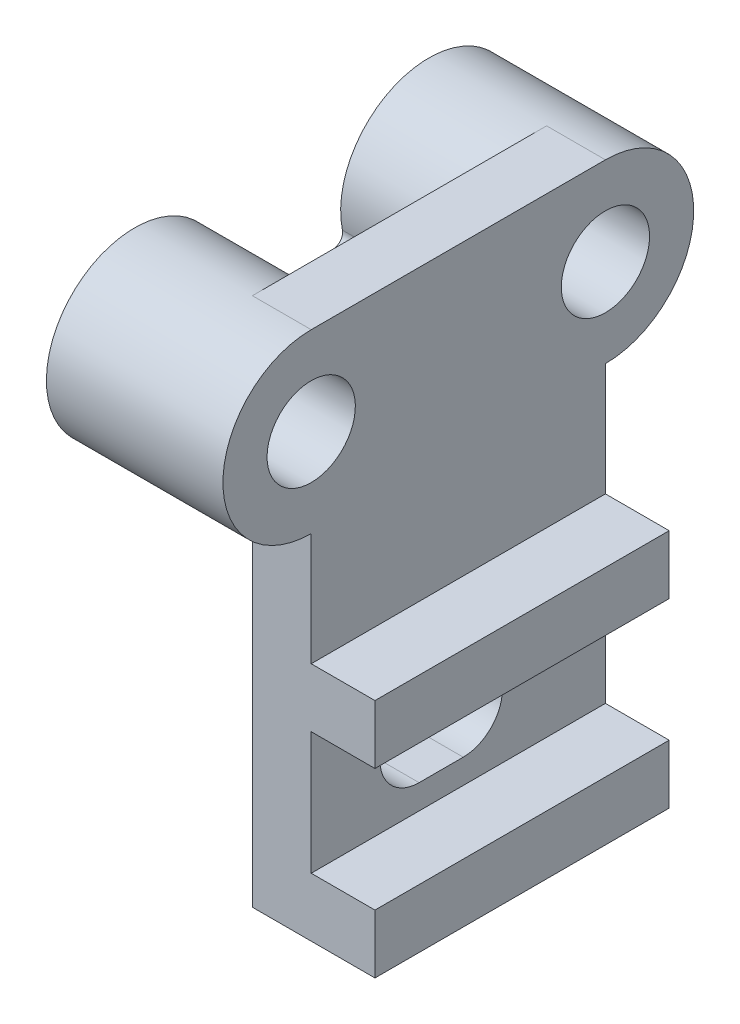
ISO-10303-21;
HEADER;
FILE_DESCRIPTION(('STEP AP214'),'2;1');
FILE_NAME('part.step','',(''),(''),'','','');
FILE_SCHEMA(('AUTOMOTIVE_DESIGN { 1 0 10303 214 1 1 1 1 }'));
ENDSEC;
DATA;
#1=APPLICATION_CONTEXT('core data for automotive mechanical design processes');
#2=APPLICATION_PROTOCOL_DEFINITION('international standard','automotive_design',2000,#1);
#3=PRODUCT_CONTEXT('',#1,'mechanical');
#4=PRODUCT('Part','Part','',(#3));
#5=PRODUCT_RELATED_PRODUCT_CATEGORY('part','',(#4));
#6=PRODUCT_DEFINITION_FORMATION('','',#4);
#7=PRODUCT_DEFINITION_CONTEXT('part definition',#1,'design');
#8=PRODUCT_DEFINITION('design','',#6,#7);
#9=PRODUCT_DEFINITION_SHAPE('','',#8);
#10=(LENGTH_UNIT() NAMED_UNIT(*) SI_UNIT(.MILLI.,.METRE.));
#11=(NAMED_UNIT(*) PLANE_ANGLE_UNIT() SI_UNIT($,.RADIAN.));
#12=(NAMED_UNIT(*) SI_UNIT($,.STERADIAN.) SOLID_ANGLE_UNIT());
#13=UNCERTAINTY_MEASURE_WITH_UNIT(LENGTH_MEASURE(1.E-05),#10,'distance_accuracy_value','');
#14=(GEOMETRIC_REPRESENTATION_CONTEXT(3) GLOBAL_UNCERTAINTY_ASSIGNED_CONTEXT((#13)) GLOBAL_UNIT_ASSIGNED_CONTEXT((#10,
#11,#12)) REPRESENTATION_CONTEXT('',''));
#15=CARTESIAN_POINT('',(0.,0.,0.));
#16=DIRECTION('',(0.,0.,1.));
#17=DIRECTION('',(1.,0.,0.));
#18=AXIS2_PLACEMENT_3D('',#15,#16,#17);
#19=CARTESIAN_POINT('',(0.,0.,30.));
#20=DIRECTION('',(1.,0.,0.));
#21=DIRECTION('',(0.,0.,-1.));
#22=AXIS2_PLACEMENT_3D('',#19,#20,#21);
#23=PLANE('',#22);
#24=DIRECTION('',(0.,0.,1.));
#25=VECTOR('',#24,1.);
#26=CARTESIAN_POINT('',(0.,17.,-0.999999999999999));
#27=LINE('',#26,#25);
#28=CARTESIAN_POINT('',(0.,17.,-0.999999999999997));
#29=VERTEX_POINT('',#28);
#30=CARTESIAN_POINT('',(0.,17.,8.));
#31=VERTEX_POINT('',#30);
#32=EDGE_CURVE('E207',#29,#31,#27,.T.);
#33=ORIENTED_EDGE('',*,*,#32,.F.);
#34=CARTESIAN_POINT('',(0.,25.,-0.999999999999999));
#35=DIRECTION('',(-1.,0.,0.));
#36=DIRECTION('',(0.,0.,1.));
#37=AXIS2_PLACEMENT_3D('',#34,#35,#36);
#38=CIRCLE('',#37,8.);
#39=CARTESIAN_POINT('',(0.,33.,-0.999999999999999));
#40=VERTEX_POINT('',#39);
#41=EDGE_CURVE('E53',#40,#29,#38,.T.);
#42=ORIENTED_EDGE('',*,*,#41,.F.);
#43=DIRECTION('',(0.,0.,-1.));
#44=VECTOR('',#43,1.);
#45=CARTESIAN_POINT('',(0.,33.,-0.999999999999999));
#46=LINE('',#45,#44);
#47=CARTESIAN_POINT('',(0.,33.,8.));
#48=VERTEX_POINT('',#47);
#49=EDGE_CURVE('E194',#48,#40,#46,.T.);
#50=ORIENTED_EDGE('',*,*,#49,.F.);
#51=CARTESIAN_POINT('',(0.,25.,8.));
#52=DIRECTION('',(-1.,0.,0.));
#53=DIRECTION('',(0.,0.,1.));
#54=AXIS2_PLACEMENT_3D('',#51,#52,#53);
#55=CIRCLE('',#54,8.);
#56=EDGE_CURVE('E214',#31,#48,#55,.T.);
#57=ORIENTED_EDGE('',*,*,#56,.F.);
#58=EDGE_LOOP('',(#33,#42,#50,#57));
#59=FACE_BOUND('',#58,.T.);
#60=DIRECTION('',(0.,1.,0.));
#61=VECTOR('',#60,1.);
#62=CARTESIAN_POINT('',(0.,0.,-18.));
#63=LINE('',#62,#61);
#64=CARTESIAN_POINT('',(0.,0.,-18.));
#65=VERTEX_POINT('',#64);
#66=CARTESIAN_POINT('',(0.,72.,-18.));
#67=VERTEX_POINT('',#66);
#68=EDGE_CURVE('E248',#65,#67,#63,.T.);
#69=ORIENTED_EDGE('',*,*,#68,.F.);
#70=DIRECTION('',(0.,0.,-1.));
#71=VECTOR('',#70,1.);
#72=CARTESIAN_POINT('',(0.,0.,30.));
#73=LINE('',#72,#71);
#74=CARTESIAN_POINT('',(0.,0.,30.));
#75=VERTEX_POINT('',#74);
#76=EDGE_CURVE('E296',#75,#65,#73,.T.);
#77=ORIENTED_EDGE('',*,*,#76,.F.);
#78=DIRECTION('',(0.,-1.,0.));
#79=VECTOR('',#78,1.);
#80=CARTESIAN_POINT('',(0.,0.,30.));
#81=LINE('',#80,#79);
#82=CARTESIAN_POINT('',(0.,72.,30.));
#83=VERTEX_POINT('',#82);
#84=EDGE_CURVE('E299',#83,#75,#81,.T.);
#85=ORIENTED_EDGE('',*,*,#84,.F.);
#86=DIRECTION('',(0.,0.,1.));
#87=VECTOR('',#86,1.);
#88=CARTESIAN_POINT('',(0.,72.,30.));
#89=LINE('',#88,#87);
#90=EDGE_CURVE('E268',#67,#83,#89,.T.);
#91=ORIENTED_EDGE('',*,*,#90,.F.);
#92=EDGE_LOOP('',(#69,#77,#85,#91));
#93=FACE_BOUND('',#92,.T.);
#94=ADVANCED_FACE('F39',(#59,#93),#23,.F.);
#95=CARTESIAN_POINT('',(-24.,72.,-30.));
#96=DIRECTION('',(0.,1.,0.));
#97=DIRECTION('',(-1.,0.,0.));
#98=AXIS2_PLACEMENT_3D('',#95,#96,#97);
#99=PLANE('',#98);
#100=DIRECTION('',(-1.,0.,0.));
#101=VECTOR('',#100,1.);
#102=CARTESIAN_POINT('',(-24.,72.,-18.));
#103=LINE('',#102,#101);
#104=CARTESIAN_POINT('',(-24.,72.,-18.));
#105=VERTEX_POINT('',#104);
#106=EDGE_CURVE('E245',#67,#105,#103,.T.);
#107=ORIENTED_EDGE('',*,*,#106,.F.);
#108=ORIENTED_EDGE('',*,*,#90,.T.);
#109=DIRECTION('',(1.,0.,0.));
#110=VECTOR('',#109,1.);
#111=CARTESIAN_POINT('',(-24.,72.,30.));
#112=LINE('',#111,#110);
#113=CARTESIAN_POINT('',(-24.,72.,30.));
#114=VERTEX_POINT('',#113);
#115=EDGE_CURVE('E264',#114,#83,#112,.T.);
#116=ORIENTED_EDGE('',*,*,#115,.F.);
#117=DIRECTION('',(0.,0.,1.));
#118=VECTOR('',#117,1.);
#119=CARTESIAN_POINT('',(-24.,72.,-30.));
#120=LINE('',#119,#118);
#121=EDGE_CURVE('E256',#105,#114,#120,.T.);
#122=ORIENTED_EDGE('',*,*,#121,.F.);
#123=EDGE_LOOP('',(#107,#108,#116,#122));
#124=FACE_BOUND('',#123,.T.);
#125=ADVANCED_FACE('F424',(#124),#99,.F.);
#126=DIRECTION('',(0.,0.,-1.));
#127=VECTOR('',#126,1.);
#128=CARTESIAN_POINT('',(0.,84.,30.));
#129=LINE('',#128,#127);
#130=CARTESIAN_POINT('',(0.,84.,10.4040820577346));
#131=VERTEX_POINT('',#130);
#132=CARTESIAN_POINT('',(0.,84.,-10.4040820577346));
#133=VERTEX_POINT('',#132);
#134=EDGE_CURVE('E349',#131,#133,#129,.T.);
#135=ORIENTED_EDGE('',*,*,#134,.F.);
#136=CARTESIAN_POINT('',(0.,86.,10.4040820577346));
#137=DIRECTION('',(1.,0.,0.));
#138=DIRECTION('',(0.,0.,-1.));
#139=AXIS2_PLACEMENT_3D('',#136,#137,#138);
#140=CIRCLE('',#139,2.);
#141=CARTESIAN_POINT('',(0.,86.4,12.3636738519611));
#142=VERTEX_POINT('',#141);
#143=EDGE_CURVE('E357',#131,#142,#140,.F.);
#144=ORIENTED_EDGE('',*,*,#143,.T.);
#145=CARTESIAN_POINT('',(0.,90.,30.));
#146=DIRECTION('',(1.,0.,0.));
#147=DIRECTION('',(0.,0.,-1.));
#148=AXIS2_PLACEMENT_3D('',#145,#146,#147);
#149=CIRCLE('',#148,18.);
#150=CARTESIAN_POINT('',(0.,108.,30.));
#151=VERTEX_POINT('',#150);
#152=EDGE_CURVE('E275',#151,#142,#149,.F.);
#153=ORIENTED_EDGE('',*,*,#152,.F.);
#154=DIRECTION('',(0.,0.,-1.));
#155=VECTOR('',#154,1.);
#156=CARTESIAN_POINT('',(0.,108.,30.));
#157=LINE('',#156,#155);
#158=CARTESIAN_POINT('',(0.,108.,-30.));
#159=VERTEX_POINT('',#158);
#160=EDGE_CURVE('E330',#151,#159,#157,.T.);
#161=ORIENTED_EDGE('',*,*,#160,.T.);
#162=CARTESIAN_POINT('',(0.,90.,-30.));
#163=DIRECTION('',(1.,0.,0.));
#164=DIRECTION('',(0.,0.,-1.));
#165=AXIS2_PLACEMENT_3D('',#162,#163,#164);
#166=CIRCLE('',#165,18.);
#167=CARTESIAN_POINT('',(0.,86.4,-12.3636738519611));
#168=VERTEX_POINT('',#167);
#169=EDGE_CURVE('E269',#168,#159,#166,.F.);
#170=ORIENTED_EDGE('',*,*,#169,.F.);
#171=CARTESIAN_POINT('',(0.,86.,-10.4040820577346));
#172=DIRECTION('',(1.,0.,0.));
#173=DIRECTION('',(0.,0.,-1.));
#174=AXIS2_PLACEMENT_3D('',#171,#172,#173);
#175=CIRCLE('',#174,2.);
#176=EDGE_CURVE('E360',#168,#133,#175,.F.);
#177=ORIENTED_EDGE('',*,*,#176,.T.);
#178=EDGE_LOOP('',(#135,#144,#153,#161,#170,#177));
#179=FACE_BOUND('',#178,.T.);
#180=ADVANCED_FACE('F381',(#179),#23,.F.);
#181=CARTESIAN_POINT('',(0.,0.,30.));
#182=DIRECTION('',(0.,0.,-1.));
#183=DIRECTION('',(-1.,0.,0.));
#184=AXIS2_PLACEMENT_3D('',#181,#182,#183);
#185=PLANE('',#184);
#186=CARTESIAN_POINT('',(12.,72.,30.));
#187=VERTEX_POINT('',#186);
#188=EDGE_CURVE('E265',#83,#187,#112,.T.);
#189=ORIENTED_EDGE('',*,*,#188,.F.);
#190=ORIENTED_EDGE('',*,*,#84,.T.);
#191=DIRECTION('',(1.,0.,0.));
#192=VECTOR('',#191,1.);
#193=CARTESIAN_POINT('',(25.,0.,30.));
#194=LINE('',#193,#192);
#195=CARTESIAN_POINT('',(25.,0.,30.));
#196=VERTEX_POINT('',#195);
#197=EDGE_CURVE('E277',#75,#196,#194,.T.);
#198=ORIENTED_EDGE('',*,*,#197,.T.);
#199=DIRECTION('',(0.,1.,0.));
#200=VECTOR('',#199,1.);
#201=CARTESIAN_POINT('',(25.,12.,30.));
#202=LINE('',#201,#200);
#203=CARTESIAN_POINT('',(25.,12.,30.));
#204=VERTEX_POINT('',#203);
#205=EDGE_CURVE('E276',#196,#204,#202,.T.);
#206=ORIENTED_EDGE('',*,*,#205,.T.);
#207=DIRECTION('',(-1.,0.,0.));
#208=VECTOR('',#207,1.);
#209=CARTESIAN_POINT('',(12.,12.,30.));
#210=LINE('',#209,#208);
#211=CARTESIAN_POINT('',(12.,12.,30.));
#212=VERTEX_POINT('',#211);
#213=EDGE_CURVE('E284',#204,#212,#210,.T.);
#214=ORIENTED_EDGE('',*,*,#213,.T.);
#215=DIRECTION('',(0.,1.,0.));
#216=VECTOR('',#215,1.);
#217=CARTESIAN_POINT('',(12.,37.,30.));
#218=LINE('',#217,#216);
#219=CARTESIAN_POINT('',(12.,37.,30.));
#220=VERTEX_POINT('',#219);
#221=EDGE_CURVE('E281',#212,#220,#218,.T.);
#222=ORIENTED_EDGE('',*,*,#221,.T.);
#223=DIRECTION('',(1.,0.,0.));
#224=VECTOR('',#223,1.);
#225=CARTESIAN_POINT('',(25.,37.,30.));
#226=LINE('',#225,#224);
#227=CARTESIAN_POINT('',(25.,37.,30.));
#228=VERTEX_POINT('',#227);
#229=EDGE_CURVE('E288',#220,#228,#226,.T.);
#230=ORIENTED_EDGE('',*,*,#229,.T.);
#231=DIRECTION('',(0.,1.,0.));
#232=VECTOR('',#231,1.);
#233=CARTESIAN_POINT('',(25.,49.,30.));
#234=LINE('',#233,#232);
#235=CARTESIAN_POINT('',(25.,49.,30.));
#236=VERTEX_POINT('',#235);
#237=EDGE_CURVE('E286',#228,#236,#234,.T.);
#238=ORIENTED_EDGE('',*,*,#237,.T.);
#239=DIRECTION('',(-1.,0.,0.));
#240=VECTOR('',#239,1.);
#241=CARTESIAN_POINT('',(12.,49.,30.));
#242=LINE('',#241,#240);
#243=CARTESIAN_POINT('',(12.,49.,30.));
#244=VERTEX_POINT('',#243);
#245=EDGE_CURVE('E289',#236,#244,#242,.T.);
#246=ORIENTED_EDGE('',*,*,#245,.T.);
#247=DIRECTION('',(0.,1.,0.));
#248=VECTOR('',#247,1.);
#249=CARTESIAN_POINT('',(12.,108.,30.));
#250=LINE('',#249,#248);
#251=EDGE_CURVE('E295',#244,#187,#250,.T.);
#252=ORIENTED_EDGE('',*,*,#251,.T.);
#253=EDGE_LOOP('',(#189,#190,#198,#206,#214,#222,#230,#238,#246,#252));
#254=FACE_BOUND('',#253,.T.);
#255=ADVANCED_FACE('F430',(#254),#185,.F.);
#256=CARTESIAN_POINT('',(0.,0.,-30.));
#257=DIRECTION('',(0.,0.,-1.));
#258=DIRECTION('',(-1.,0.,0.));
#259=AXIS2_PLACEMENT_3D('',#256,#257,#258);
#260=PLANE('',#259);
#261=DIRECTION('',(1.,0.,0.));
#262=VECTOR('',#261,1.);
#263=CARTESIAN_POINT('',(25.,0.,-30.));
#264=LINE('',#263,#262);
#265=CARTESIAN_POINT('',(0.,0.,-30.));
#266=VERTEX_POINT('',#265);
#267=CARTESIAN_POINT('',(25.,0.,-30.));
#268=VERTEX_POINT('',#267);
#269=EDGE_CURVE('E274',#266,#268,#264,.T.);
#270=ORIENTED_EDGE('',*,*,#269,.F.);
#271=DIRECTION('',(-0.316227766016838,0.948683298050514,0.));
#272=VECTOR('',#271,1.);
#273=CARTESIAN_POINT('',(-24.,72.,-30.));
#274=LINE('',#273,#272);
#275=CARTESIAN_POINT('',(-24.,72.,-30.));
#276=VERTEX_POINT('',#275);
#277=EDGE_CURVE('E237',#266,#276,#274,.T.);
#278=ORIENTED_EDGE('',*,*,#277,.T.);
#279=DIRECTION('',(1.,0.,0.));
#280=VECTOR('',#279,1.);
#281=CARTESIAN_POINT('',(0.,72.,-30.));
#282=LINE('',#281,#280);
#283=CARTESIAN_POINT('',(12.,72.,-30.));
#284=VERTEX_POINT('',#283);
#285=EDGE_CURVE('E347',#276,#284,#282,.T.);
#286=ORIENTED_EDGE('',*,*,#285,.T.);
#287=DIRECTION('',(0.,1.,0.));
#288=VECTOR('',#287,1.);
#289=CARTESIAN_POINT('',(12.,108.,-30.));
#290=LINE('',#289,#288);
#291=CARTESIAN_POINT('',(12.,49.,-30.));
#292=VERTEX_POINT('',#291);
#293=EDGE_CURVE('E319',#292,#284,#290,.T.);
#294=ORIENTED_EDGE('',*,*,#293,.F.);
#295=DIRECTION('',(-1.,0.,0.));
#296=VECTOR('',#295,1.);
#297=CARTESIAN_POINT('',(12.,49.,-30.));
#298=LINE('',#297,#296);
#299=CARTESIAN_POINT('',(25.,49.,-30.));
#300=VERTEX_POINT('',#299);
#301=EDGE_CURVE('E320',#300,#292,#298,.T.);
#302=ORIENTED_EDGE('',*,*,#301,.F.);
#303=DIRECTION('',(0.,1.,0.));
#304=VECTOR('',#303,1.);
#305=CARTESIAN_POINT('',(25.,49.,-30.));
#306=LINE('',#305,#304);
#307=CARTESIAN_POINT('',(25.,37.,-30.));
#308=VERTEX_POINT('',#307);
#309=EDGE_CURVE('E314',#308,#300,#306,.T.);
#310=ORIENTED_EDGE('',*,*,#309,.F.);
#311=DIRECTION('',(1.,0.,0.));
#312=VECTOR('',#311,1.);
#313=CARTESIAN_POINT('',(25.,37.,-30.));
#314=LINE('',#313,#312);
#315=CARTESIAN_POINT('',(12.,37.,-30.));
#316=VERTEX_POINT('',#315);
#317=EDGE_CURVE('E313',#316,#308,#314,.T.);
#318=ORIENTED_EDGE('',*,*,#317,.F.);
#319=DIRECTION('',(0.,1.,0.));
#320=VECTOR('',#319,1.);
#321=CARTESIAN_POINT('',(12.,37.,-30.));
#322=LINE('',#321,#320);
#323=CARTESIAN_POINT('',(12.,12.,-30.));
#324=VERTEX_POINT('',#323);
#325=EDGE_CURVE('E306',#324,#316,#322,.T.);
#326=ORIENTED_EDGE('',*,*,#325,.F.);
#327=DIRECTION('',(-1.,0.,0.));
#328=VECTOR('',#327,1.);
#329=CARTESIAN_POINT('',(12.,12.,-30.));
#330=LINE('',#329,#328);
#331=CARTESIAN_POINT('',(25.,12.,-30.));
#332=VERTEX_POINT('',#331);
#333=EDGE_CURVE('E304',#332,#324,#330,.T.);
#334=ORIENTED_EDGE('',*,*,#333,.F.);
#335=DIRECTION('',(0.,1.,0.));
#336=VECTOR('',#335,1.);
#337=CARTESIAN_POINT('',(25.,12.,-30.));
#338=LINE('',#337,#336);
#339=EDGE_CURVE('E305',#268,#332,#338,.T.);
#340=ORIENTED_EDGE('',*,*,#339,.F.);
#341=EDGE_LOOP('',(#270,#278,#286,#294,#302,#310,#318,#326,#334,#340));
#342=FACE_BOUND('',#341,.T.);
#343=ADVANCED_FACE('F407',(#342),#260,.T.);
#344=CARTESIAN_POINT('',(25.,0.,30.));
#345=DIRECTION('',(0.,1.,0.));
#346=DIRECTION('',(-1.,0.,0.));
#347=AXIS2_PLACEMENT_3D('',#344,#345,#346);
#348=PLANE('',#347);
#349=ORIENTED_EDGE('',*,*,#269,.T.);
#350=DIRECTION('',(0.,0.,-1.));
#351=VECTOR('',#350,1.);
#352=CARTESIAN_POINT('',(25.,0.,30.));
#353=LINE('',#352,#351);
#354=EDGE_CURVE('E342',#196,#268,#353,.T.);
#355=ORIENTED_EDGE('',*,*,#354,.F.);
#356=ORIENTED_EDGE('',*,*,#197,.F.);
#357=ORIENTED_EDGE('',*,*,#76,.T.);
#358=DIRECTION('',(0.,0.,-1.));
#359=VECTOR('',#358,1.);
#360=CARTESIAN_POINT('',(0.,0.,-30.));
#361=LINE('',#360,#359);
#362=EDGE_CURVE('E239',#65,#266,#361,.T.);
#363=ORIENTED_EDGE('',*,*,#362,.T.);
#364=EDGE_LOOP('',(#349,#355,#356,#357,#363));
#365=FACE_BOUND('',#364,.T.);
#366=ADVANCED_FACE('F413',(#365),#348,.F.);
#367=CARTESIAN_POINT('',(25.,12.,30.));
#368=DIRECTION('',(-1.,0.,0.));
#369=DIRECTION('',(0.,-1.,0.));
#370=AXIS2_PLACEMENT_3D('',#367,#368,#369);
#371=PLANE('',#370);
#372=ORIENTED_EDGE('',*,*,#339,.T.);
#373=DIRECTION('',(0.,0.,-1.));
#374=VECTOR('',#373,1.);
#375=CARTESIAN_POINT('',(25.,12.,30.));
#376=LINE('',#375,#374);
#377=EDGE_CURVE('E345',#204,#332,#376,.T.);
#378=ORIENTED_EDGE('',*,*,#377,.F.);
#379=ORIENTED_EDGE('',*,*,#205,.F.);
#380=ORIENTED_EDGE('',*,*,#354,.T.);
#381=EDGE_LOOP('',(#372,#378,#379,#380));
#382=FACE_BOUND('',#381,.T.);
#383=ADVANCED_FACE('F454',(#382),#371,.F.);
#384=CARTESIAN_POINT('',(12.,12.,30.));
#385=DIRECTION('',(0.,-1.,0.));
#386=DIRECTION('',(0.,0.,-1.));
#387=AXIS2_PLACEMENT_3D('',#384,#385,#386);
#388=PLANE('',#387);
#389=ORIENTED_EDGE('',*,*,#333,.T.);
#390=DIRECTION('',(0.,0.,-1.));
#391=VECTOR('',#390,1.);
#392=CARTESIAN_POINT('',(12.,12.,30.));
#393=LINE('',#392,#391);
#394=EDGE_CURVE('E338',#212,#324,#393,.T.);
#395=ORIENTED_EDGE('',*,*,#394,.F.);
#396=ORIENTED_EDGE('',*,*,#213,.F.);
#397=ORIENTED_EDGE('',*,*,#377,.T.);
#398=EDGE_LOOP('',(#389,#395,#396,#397));
#399=FACE_BOUND('',#398,.T.);
#400=ADVANCED_FACE('F455',(#399),#388,.F.);
#401=CARTESIAN_POINT('',(12.,37.,30.));
#402=DIRECTION('',(-1.,0.,0.));
#403=DIRECTION('',(0.,-1.,0.));
#404=AXIS2_PLACEMENT_3D('',#401,#402,#403);
#405=PLANE('',#404);
#406=DIRECTION('',(0.,0.,1.));
#407=VECTOR('',#406,1.);
#408=CARTESIAN_POINT('',(12.,33.,-0.999999999999999));
#409=LINE('',#408,#407);
#410=CARTESIAN_POINT('',(12.,33.,-0.999999999999999));
#411=VERTEX_POINT('',#410);
#412=CARTESIAN_POINT('',(12.,33.,8.));
#413=VERTEX_POINT('',#412);
#414=EDGE_CURVE('E210',#411,#413,#409,.T.);
#415=ORIENTED_EDGE('',*,*,#414,.F.);
#416=CARTESIAN_POINT('',(12.,25.,-0.999999999999999));
#417=DIRECTION('',(-1.,0.,0.));
#418=DIRECTION('',(0.,-1.,0.));
#419=AXIS2_PLACEMENT_3D('',#416,#417,#418);
#420=CIRCLE('',#419,8.);
#421=CARTESIAN_POINT('',(12.,17.,-0.999999999999999));
#422=VERTEX_POINT('',#421);
#423=EDGE_CURVE('E186',#422,#411,#420,.F.);
#424=ORIENTED_EDGE('',*,*,#423,.F.);
#425=DIRECTION('',(0.,0.,-1.));
#426=VECTOR('',#425,1.);
#427=CARTESIAN_POINT('',(12.,17.,-0.999999999999999));
#428=LINE('',#427,#426);
#429=CARTESIAN_POINT('',(12.,17.,8.));
#430=VERTEX_POINT('',#429);
#431=EDGE_CURVE('E196',#430,#422,#428,.T.);
#432=ORIENTED_EDGE('',*,*,#431,.F.);
#433=CARTESIAN_POINT('',(12.,25.,8.));
#434=DIRECTION('',(-1.,0.,0.));
#435=DIRECTION('',(0.,-1.,0.));
#436=AXIS2_PLACEMENT_3D('',#433,#434,#435);
#437=CIRCLE('',#436,8.);
#438=EDGE_CURVE('E64',#413,#430,#437,.F.);
#439=ORIENTED_EDGE('',*,*,#438,.F.);
#440=EDGE_LOOP('',(#415,#424,#432,#439));
#441=FACE_BOUND('',#440,.T.);
#442=ORIENTED_EDGE('',*,*,#325,.T.);
#443=DIRECTION('',(0.,0.,-1.));
#444=VECTOR('',#443,1.);
#445=CARTESIAN_POINT('',(12.,37.,30.));
#446=LINE('',#445,#444);
#447=EDGE_CURVE('E340',#220,#316,#446,.T.);
#448=ORIENTED_EDGE('',*,*,#447,.F.);
#449=ORIENTED_EDGE('',*,*,#221,.F.);
#450=ORIENTED_EDGE('',*,*,#394,.T.);
#451=EDGE_LOOP('',(#442,#448,#449,#450));
#452=FACE_BOUND('',#451,.T.);
#453=ADVANCED_FACE('F204',(#441,#452),#405,.F.);
#454=CARTESIAN_POINT('',(25.,37.,30.));
#455=DIRECTION('',(0.,1.,0.));
#456=DIRECTION('',(-1.,0.,0.));
#457=AXIS2_PLACEMENT_3D('',#454,#455,#456);
#458=PLANE('',#457);
#459=ORIENTED_EDGE('',*,*,#317,.T.);
#460=DIRECTION('',(0.,0.,-1.));
#461=VECTOR('',#460,1.);
#462=CARTESIAN_POINT('',(25.,37.,30.));
#463=LINE('',#462,#461);
#464=EDGE_CURVE('E337',#228,#308,#463,.T.);
#465=ORIENTED_EDGE('',*,*,#464,.F.);
#466=ORIENTED_EDGE('',*,*,#229,.F.);
#467=ORIENTED_EDGE('',*,*,#447,.T.);
#468=EDGE_LOOP('',(#459,#465,#466,#467));
#469=FACE_BOUND('',#468,.T.);
#470=ADVANCED_FACE('F443',(#469),#458,.F.);
#471=CARTESIAN_POINT('',(25.,49.,30.));
#472=DIRECTION('',(-1.,0.,0.));
#473=DIRECTION('',(0.,0.,1.));
#474=AXIS2_PLACEMENT_3D('',#471,#472,#473);
#475=PLANE('',#474);
#476=ORIENTED_EDGE('',*,*,#309,.T.);
#477=DIRECTION('',(0.,0.,-1.));
#478=VECTOR('',#477,1.);
#479=CARTESIAN_POINT('',(25.,49.,30.));
#480=LINE('',#479,#478);
#481=EDGE_CURVE('E331',#236,#300,#480,.T.);
#482=ORIENTED_EDGE('',*,*,#481,.F.);
#483=ORIENTED_EDGE('',*,*,#237,.F.);
#484=ORIENTED_EDGE('',*,*,#464,.T.);
#485=EDGE_LOOP('',(#476,#482,#483,#484));
#486=FACE_BOUND('',#485,.T.);
#487=ADVANCED_FACE('F442',(#486),#475,.F.);
#488=CARTESIAN_POINT('',(12.,49.,30.));
#489=DIRECTION('',(0.,-1.,0.));
#490=DIRECTION('',(0.,0.,-1.));
#491=AXIS2_PLACEMENT_3D('',#488,#489,#490);
#492=PLANE('',#491);
#493=ORIENTED_EDGE('',*,*,#301,.T.);
#494=DIRECTION('',(0.,0.,-1.));
#495=VECTOR('',#494,1.);
#496=CARTESIAN_POINT('',(12.,49.,30.));
#497=LINE('',#496,#495);
#498=EDGE_CURVE('E335',#244,#292,#497,.T.);
#499=ORIENTED_EDGE('',*,*,#498,.F.);
#500=ORIENTED_EDGE('',*,*,#245,.F.);
#501=ORIENTED_EDGE('',*,*,#481,.T.);
#502=EDGE_LOOP('',(#493,#499,#500,#501));
#503=FACE_BOUND('',#502,.T.);
#504=ADVANCED_FACE('F440',(#503),#492,.F.);
#505=CARTESIAN_POINT('',(12.,108.,30.));
#506=DIRECTION('',(-1.,0.,0.));
#507=DIRECTION('',(0.,-1.,0.));
#508=AXIS2_PLACEMENT_3D('',#505,#506,#507);
#509=PLANE('',#508);
#510=CARTESIAN_POINT('',(12.,90.,-30.));
#511=DIRECTION('',(-1.,0.,0.));
#512=DIRECTION('',(0.,-1.,0.));
#513=AXIS2_PLACEMENT_3D('',#510,#511,#512);
#514=CIRCLE('',#513,9.00000000000001);
#515=CARTESIAN_POINT('',(12.,81.,-30.));
#516=VERTEX_POINT('',#515);
#517=EDGE_CURVE('E229',#516,#516,#514,.F.);
#518=ORIENTED_EDGE('',*,*,#517,.F.);
#519=EDGE_LOOP('',(#518));
#520=FACE_BOUND('',#519,.T.);
#521=CARTESIAN_POINT('',(12.,90.,30.));
#522=DIRECTION('',(-1.,0.,0.));
#523=DIRECTION('',(0.,-1.,0.));
#524=AXIS2_PLACEMENT_3D('',#521,#522,#523);
#525=CIRCLE('',#524,9.00000000000001);
#526=CARTESIAN_POINT('',(12.,81.,30.));
#527=VERTEX_POINT('',#526);
#528=EDGE_CURVE('E230',#527,#527,#525,.F.);
#529=ORIENTED_EDGE('',*,*,#528,.F.);
#530=EDGE_LOOP('',(#529));
#531=FACE_BOUND('',#530,.T.);
#532=CARTESIAN_POINT('',(12.,90.,-30.));
#533=DIRECTION('',(-1.,0.,0.));
#534=DIRECTION('',(0.,-1.,0.));
#535=AXIS2_PLACEMENT_3D('',#532,#533,#534);
#536=CIRCLE('',#535,18.);
#537=CARTESIAN_POINT('',(12.,108.,-30.));
#538=VERTEX_POINT('',#537);
#539=EDGE_CURVE('E251',#538,#284,#536,.T.);
#540=ORIENTED_EDGE('',*,*,#539,.F.);
#541=DIRECTION('',(0.,0.,-1.));
#542=VECTOR('',#541,1.);
#543=CARTESIAN_POINT('',(12.,108.,30.));
#544=LINE('',#543,#542);
#545=CARTESIAN_POINT('',(12.,108.,30.));
#546=VERTEX_POINT('',#545);
#547=EDGE_CURVE('E329',#546,#538,#544,.T.);
#548=ORIENTED_EDGE('',*,*,#547,.F.);
#549=CARTESIAN_POINT('',(12.,90.,30.));
#550=DIRECTION('',(-1.,0.,0.));
#551=DIRECTION('',(0.,-1.,0.));
#552=AXIS2_PLACEMENT_3D('',#549,#550,#551);
#553=CIRCLE('',#552,18.);
#554=EDGE_CURVE('E246',#187,#546,#553,.T.);
#555=ORIENTED_EDGE('',*,*,#554,.F.);
#556=ORIENTED_EDGE('',*,*,#251,.F.);
#557=ORIENTED_EDGE('',*,*,#498,.T.);
#558=ORIENTED_EDGE('',*,*,#293,.T.);
#559=EDGE_LOOP('',(#540,#548,#555,#556,#557,#558));
#560=FACE_BOUND('',#559,.T.);
#561=ADVANCED_FACE('F435',(#520,#531,#560),#509,.F.);
#562=CARTESIAN_POINT('',(0.,108.,30.));
#563=DIRECTION('',(0.,-1.,0.));
#564=DIRECTION('',(0.,0.,-1.));
#565=AXIS2_PLACEMENT_3D('',#562,#563,#564);
#566=PLANE('',#565);
#567=DIRECTION('',(-1.,0.,0.));
#568=VECTOR('',#567,1.);
#569=CARTESIAN_POINT('',(0.,108.,-30.));
#570=LINE('',#569,#568);
#571=EDGE_CURVE('E278',#538,#159,#570,.T.);
#572=ORIENTED_EDGE('',*,*,#571,.T.);
#573=ORIENTED_EDGE('',*,*,#160,.F.);
#574=DIRECTION('',(-1.,0.,0.));
#575=VECTOR('',#574,1.);
#576=CARTESIAN_POINT('',(0.,108.,30.));
#577=LINE('',#576,#575);
#578=EDGE_CURVE('E293',#546,#151,#577,.T.);
#579=ORIENTED_EDGE('',*,*,#578,.F.);
#580=ORIENTED_EDGE('',*,*,#547,.T.);
#581=EDGE_LOOP('',(#572,#573,#579,#580));
#582=FACE_BOUND('',#581,.T.);
#583=ADVANCED_FACE('F386',(#582),#566,.F.);
#584=CARTESIAN_POINT('',(-24.,84.,-13.0294372515229));
#585=DIRECTION('',(0.,-1.,0.));
#586=DIRECTION('',(1.,0.,0.));
#587=AXIS2_PLACEMENT_3D('',#584,#585,#586);
#588=PLANE('',#587);
#589=DIRECTION('',(0.,0.,-1.));
#590=VECTOR('',#589,1.);
#591=CARTESIAN_POINT('',(-24.,84.,-13.0294372515229));
#592=LINE('',#591,#590);
#593=CARTESIAN_POINT('',(-24.,84.,10.4040820577346));
#594=VERTEX_POINT('',#593);
#595=CARTESIAN_POINT('',(-24.,84.,-10.4040820577346));
#596=VERTEX_POINT('',#595);
#597=EDGE_CURVE('E252',#594,#596,#592,.T.);
#598=ORIENTED_EDGE('',*,*,#597,.F.);
#599=DIRECTION('',(-1.,0.,0.));
#600=VECTOR('',#599,1.);
#601=CARTESIAN_POINT('',(0.,84.,10.4040820577346));
#602=LINE('',#601,#600);
#603=EDGE_CURVE('E351',#594,#131,#602,.F.);
#604=ORIENTED_EDGE('',*,*,#603,.T.);
#605=ORIENTED_EDGE('',*,*,#134,.T.);
#606=DIRECTION('',(-1.,0.,0.));
#607=VECTOR('',#606,1.);
#608=CARTESIAN_POINT('',(-24.,84.,-10.4040820577346));
#609=LINE('',#608,#607);
#610=EDGE_CURVE('E354',#133,#596,#609,.T.);
#611=ORIENTED_EDGE('',*,*,#610,.T.);
#612=EDGE_LOOP('',(#598,#604,#605,#611));
#613=FACE_BOUND('',#612,.T.);
#614=ADVANCED_FACE('F374',(#613),#588,.F.);
#615=CARTESIAN_POINT('',(-24.,90.,30.));
#616=DIRECTION('',(1.,0.,0.));
#617=DIRECTION('',(0.,1.,0.));
#618=AXIS2_PLACEMENT_3D('',#615,#616,#617);
#619=CYLINDRICAL_SURFACE('',#618,18.);
#620=ORIENTED_EDGE('',*,*,#152,.T.);
#621=DIRECTION('',(1.,0.,0.));
#622=VECTOR('',#621,1.);
#623=CARTESIAN_POINT('',(-24.,86.4,12.3636738519611));
#624=LINE('',#623,#622);
#625=CARTESIAN_POINT('',(-24.,86.4,12.3636738519611));
#626=VERTEX_POINT('',#625);
#627=EDGE_CURVE('E363',#142,#626,#624,.F.);
#628=ORIENTED_EDGE('',*,*,#627,.T.);
#629=CARTESIAN_POINT('',(-24.,90.,30.));
#630=DIRECTION('',(-1.,0.,0.));
#631=DIRECTION('',(0.,-1.,0.));
#632=AXIS2_PLACEMENT_3D('',#629,#630,#631);
#633=CIRCLE('',#632,18.);
#634=EDGE_CURVE('E247',#114,#626,#633,.T.);
#635=ORIENTED_EDGE('',*,*,#634,.F.);
#636=ORIENTED_EDGE('',*,*,#115,.T.);
#637=ORIENTED_EDGE('',*,*,#188,.T.);
#638=ORIENTED_EDGE('',*,*,#554,.T.);
#639=ORIENTED_EDGE('',*,*,#578,.T.);
#640=EDGE_LOOP('',(#620,#628,#635,#636,#637,#638,#639));
#641=FACE_BOUND('',#640,.T.);
#642=ADVANCED_FACE('F383',(#641),#619,.T.);
#643=CARTESIAN_POINT('',(-24.,90.,-30.));
#644=DIRECTION('',(1.,0.,0.));
#645=DIRECTION('',(0.,1.,0.));
#646=AXIS2_PLACEMENT_3D('',#643,#644,#645);
#647=CYLINDRICAL_SURFACE('',#646,18.);
#648=CARTESIAN_POINT('',(-24.,90.,-30.));
#649=DIRECTION('',(-1.,0.,0.));
#650=DIRECTION('',(0.,-1.,0.));
#651=AXIS2_PLACEMENT_3D('',#648,#649,#650);
#652=CIRCLE('',#651,18.);
#653=CARTESIAN_POINT('',(-24.,86.4,-12.3636738519611));
#654=VERTEX_POINT('',#653);
#655=EDGE_CURVE('E258',#654,#276,#652,.T.);
#656=ORIENTED_EDGE('',*,*,#655,.F.);
#657=DIRECTION('',(1.,0.,0.));
#658=VECTOR('',#657,1.);
#659=CARTESIAN_POINT('',(-24.,86.4,-12.3636738519611));
#660=LINE('',#659,#658);
#661=EDGE_CURVE('E361',#654,#168,#660,.T.);
#662=ORIENTED_EDGE('',*,*,#661,.T.);
#663=ORIENTED_EDGE('',*,*,#169,.T.);
#664=ORIENTED_EDGE('',*,*,#571,.F.);
#665=ORIENTED_EDGE('',*,*,#539,.T.);
#666=ORIENTED_EDGE('',*,*,#285,.F.);
#667=EDGE_LOOP('',(#656,#662,#663,#664,#665,#666));
#668=FACE_BOUND('',#667,.T.);
#669=ADVANCED_FACE('F393',(#668),#647,.T.);
#670=CARTESIAN_POINT('',(-24.,90.,30.));
#671=DIRECTION('',(-1.,0.,0.));
#672=DIRECTION('',(0.,-1.,0.));
#673=AXIS2_PLACEMENT_3D('',#670,#671,#672);
#674=PLANE('',#673);
#675=CARTESIAN_POINT('',(-24.,90.,-30.));
#676=DIRECTION('',(-1.,0.,0.));
#677=DIRECTION('',(0.,-1.,0.));
#678=AXIS2_PLACEMENT_3D('',#675,#676,#677);
#679=CIRCLE('',#678,9.00000000000001);
#680=CARTESIAN_POINT('',(-24.,81.,-30.));
#681=VERTEX_POINT('',#680);
#682=EDGE_CURVE('E221',#681,#681,#679,.T.);
#683=ORIENTED_EDGE('',*,*,#682,.F.);
#684=EDGE_LOOP('',(#683));
#685=FACE_BOUND('',#684,.T.);
#686=CARTESIAN_POINT('',(-24.,90.,30.));
#687=DIRECTION('',(-1.,0.,0.));
#688=DIRECTION('',(0.,-1.,0.));
#689=AXIS2_PLACEMENT_3D('',#686,#687,#688);
#690=CIRCLE('',#689,9.00000000000001);
#691=CARTESIAN_POINT('',(-24.,81.,30.));
#692=VERTEX_POINT('',#691);
#693=EDGE_CURVE('E203',#692,#692,#690,.T.);
#694=ORIENTED_EDGE('',*,*,#693,.F.);
#695=EDGE_LOOP('',(#694));
#696=FACE_BOUND('',#695,.T.);
#697=ORIENTED_EDGE('',*,*,#597,.T.);
#698=CARTESIAN_POINT('',(-24.,86.,-10.4040820577346));
#699=DIRECTION('',(-1.,0.,0.));
#700=DIRECTION('',(0.,-1.,0.));
#701=AXIS2_PLACEMENT_3D('',#698,#699,#700);
#702=CIRCLE('',#701,2.);
#703=EDGE_CURVE('E11',#596,#654,#702,.F.);
#704=ORIENTED_EDGE('',*,*,#703,.T.);
#705=ORIENTED_EDGE('',*,*,#655,.T.);
#706=EDGE_CURVE('E259',#276,#105,#120,.T.);
#707=ORIENTED_EDGE('',*,*,#706,.T.);
#708=ORIENTED_EDGE('',*,*,#121,.T.);
#709=ORIENTED_EDGE('',*,*,#634,.T.);
#710=CARTESIAN_POINT('',(-24.,86.,10.4040820577346));
#711=DIRECTION('',(-1.,0.,0.));
#712=DIRECTION('',(0.,-1.,0.));
#713=AXIS2_PLACEMENT_3D('',#710,#711,#712);
#714=CIRCLE('',#713,2.);
#715=EDGE_CURVE('E50',#626,#594,#714,.F.);
#716=ORIENTED_EDGE('',*,*,#715,.T.);
#717=EDGE_LOOP('',(#697,#704,#705,#707,#708,#709,#716));
#718=FACE_BOUND('',#717,.T.);
#719=ADVANCED_FACE('F366',(#685,#696,#718),#674,.T.);
#720=CARTESIAN_POINT('',(0.5,54.,-18.));
#721=DIRECTION('',(0.,0.,-1.));
#722=DIRECTION('',(-1.,0.,0.));
#723=AXIS2_PLACEMENT_3D('',#720,#721,#722);
#724=PLANE('',#723);
#725=DIRECTION('',(-0.316227766016838,0.948683298050514,0.));
#726=VECTOR('',#725,1.);
#727=CARTESIAN_POINT('',(-24.,72.,-18.));
#728=LINE('',#727,#726);
#729=EDGE_CURVE('E233',#65,#105,#728,.T.);
#730=ORIENTED_EDGE('',*,*,#729,.F.);
#731=ORIENTED_EDGE('',*,*,#68,.T.);
#732=ORIENTED_EDGE('',*,*,#106,.T.);
#733=EDGE_LOOP('',(#730,#731,#732));
#734=FACE_BOUND('',#733,.T.);
#735=ADVANCED_FACE('F418',(#734),#724,.F.);
#736=CARTESIAN_POINT('',(-24.,72.,-30.));
#737=DIRECTION('',(-0.948683298050514,-0.316227766016838,0.));
#738=DIRECTION('',(-0.316227766016838,0.948683298050514,0.));
#739=AXIS2_PLACEMENT_3D('',#736,#737,#738);
#740=PLANE('',#739);
#741=ORIENTED_EDGE('',*,*,#362,.F.);
#742=ORIENTED_EDGE('',*,*,#729,.T.);
#743=ORIENTED_EDGE('',*,*,#706,.F.);
#744=ORIENTED_EDGE('',*,*,#277,.F.);
#745=EDGE_LOOP('',(#741,#742,#743,#744));
#746=FACE_BOUND('',#745,.T.);
#747=ADVANCED_FACE('F401',(#746),#740,.T.);
#748=CARTESIAN_POINT('',(25.001,90.,30.));
#749=DIRECTION('',(-1.,0.,0.));
#750=DIRECTION('',(0.,-1.,0.));
#751=AXIS2_PLACEMENT_3D('',#748,#749,#750);
#752=CYLINDRICAL_SURFACE('',#751,9.00000000000001);
#753=CARTESIAN_POINT('',(-24.,81.,30.));
#754=CARTESIAN_POINT('',(-23.625,81.,30.));
#755=CARTESIAN_POINT('',(-23.25,81.,30.));
#756=CARTESIAN_POINT('',(-22.5,81.,30.));
#757=CARTESIAN_POINT('',(-22.125,81.,30.));
#758=CARTESIAN_POINT('',(-21.375,81.,30.));
#759=CARTESIAN_POINT('',(-21.,81.,30.));
#760=CARTESIAN_POINT('',(-20.25,81.,30.));
#761=CARTESIAN_POINT('',(-19.875,81.,30.));
#762=CARTESIAN_POINT('',(-19.125,81.,30.));
#763=CARTESIAN_POINT('',(-18.75,81.,30.));
#764=CARTESIAN_POINT('',(-18.,81.,30.));
#765=CARTESIAN_POINT('',(-17.625,81.,30.));
#766=CARTESIAN_POINT('',(-16.875,81.,30.));
#767=CARTESIAN_POINT('',(-16.5,81.,30.));
#768=CARTESIAN_POINT('',(-15.75,81.,30.));
#769=CARTESIAN_POINT('',(-15.375,81.,30.));
#770=CARTESIAN_POINT('',(-14.625,81.,30.));
#771=CARTESIAN_POINT('',(-14.25,81.,30.));
#772=CARTESIAN_POINT('',(-13.5,81.,30.));
#773=CARTESIAN_POINT('',(-13.125,81.,30.));
#774=CARTESIAN_POINT('',(-12.375,81.,30.));
#775=CARTESIAN_POINT('',(-12.,81.,30.));
#776=CARTESIAN_POINT('',(-11.25,81.,30.));
#777=CARTESIAN_POINT('',(-10.875,81.,30.));
#778=CARTESIAN_POINT('',(-10.125,81.,30.));
#779=CARTESIAN_POINT('',(-9.75000000000001,81.,30.));
#780=CARTESIAN_POINT('',(-9.00000000000001,81.,30.));
#781=CARTESIAN_POINT('',(-8.625,81.,30.));
#782=CARTESIAN_POINT('',(-7.875,81.,30.));
#783=CARTESIAN_POINT('',(-7.5,81.,30.));
#784=CARTESIAN_POINT('',(-6.75,81.,30.));
#785=CARTESIAN_POINT('',(-6.375,81.,30.));
#786=CARTESIAN_POINT('',(-5.62500000000001,81.,30.));
#787=CARTESIAN_POINT('',(-5.25,81.,30.));
#788=CARTESIAN_POINT('',(-4.5,81.,30.));
#789=CARTESIAN_POINT('',(-4.125,81.,30.));
#790=CARTESIAN_POINT('',(-3.375,81.,30.));
#791=CARTESIAN_POINT('',(-3.,81.,30.));
#792=CARTESIAN_POINT('',(-2.25000000000001,81.,30.));
#793=CARTESIAN_POINT('',(-1.87500000000001,81.,30.));
#794=CARTESIAN_POINT('',(-1.125,81.,30.));
#795=CARTESIAN_POINT('',(-0.750000000000004,81.,30.));
#796=CARTESIAN_POINT('',(0.,81.,30.));
#797=CARTESIAN_POINT('',(0.374999999999995,81.,30.));
#798=CARTESIAN_POINT('',(1.12499999999999,81.,30.));
#799=CARTESIAN_POINT('',(1.49999999999999,81.,30.));
#800=CARTESIAN_POINT('',(2.25,81.,30.));
#801=CARTESIAN_POINT('',(2.625,81.,30.));
#802=CARTESIAN_POINT('',(3.375,81.,30.));
#803=CARTESIAN_POINT('',(3.75,81.,30.));
#804=CARTESIAN_POINT('',(4.5,81.,30.));
#805=CARTESIAN_POINT('',(4.875,81.,30.));
#806=CARTESIAN_POINT('',(5.625,81.,30.));
#807=CARTESIAN_POINT('',(6.,81.,30.));
#808=CARTESIAN_POINT('',(6.74999999999999,81.,30.));
#809=CARTESIAN_POINT('',(7.12499999999999,81.,30.));
#810=CARTESIAN_POINT('',(7.87499999999999,81.,30.));
#811=CARTESIAN_POINT('',(8.24999999999999,81.,30.));
#812=CARTESIAN_POINT('',(8.99999999999999,81.,30.));
#813=CARTESIAN_POINT('',(9.37499999999999,81.,30.));
#814=CARTESIAN_POINT('',(10.125,81.,30.));
#815=CARTESIAN_POINT('',(10.5,81.,30.));
#816=CARTESIAN_POINT('',(11.25,81.,30.));
#817=CARTESIAN_POINT('',(11.625,81.,30.));
#818=CARTESIAN_POINT('',(12.,81.,30.));
#819=B_SPLINE_CURVE_WITH_KNOTS('',3,(#753,#754,#755,#756,#757,#758,#759,#760,#761,#762,#763,
#764,#765,#766,#767,#768,#769,#770,#771,#772,#773,#774,#775,#776,#777,#778,#779,#780,#781,#782,
#783,#784,#785,#786,#787,#788,#789,#790,#791,#792,#793,#794,#795,#796,#797,#798,#799,#800,#801,
#802,#803,#804,#805,#806,#807,#808,#809,#810,#811,#812,#813,#814,#815,#816,#817,#818),
.UNSPECIFIED.,.F.,.F.,(4,2,2,2,2,2,2,2,2,2,2,2,2,2,2,2,2,2,2,2,2,2,2,2,2,2,2,2,2,2,2,2,4),(0.,
1.125,2.25,3.375,4.5,5.625,6.75,7.875,9.,10.125,11.25,12.375,13.5,14.625,15.75,16.875,18.,
19.125,20.25,21.375,22.5,23.625,24.75,25.875,27.,28.125,29.25,30.375,31.5,32.625,33.75,34.875,
36.),.UNSPECIFIED.);
#820=EDGE_CURVE('BSEAM497',#692,#527,#819,.T.);
#821=ORIENTED_EDGE('',*,*,#693,.T.);
#822=ORIENTED_EDGE('',*,*,#528,.T.);
#823=ORIENTED_EDGE('',*,*,#820,.T.);
#824=ORIENTED_EDGE('',*,*,#820,.F.);
#825=EDGE_LOOP('',(#821,#823,#822,#824));
#826=FACE_BOUND('',#825,.T.);
#827=ADVANCED_FACE('F497',(#826),#752,.F.);
#828=CARTESIAN_POINT('',(25.001,90.,-30.));
#829=DIRECTION('',(-1.,0.,0.));
#830=DIRECTION('',(0.,-1.,0.));
#831=AXIS2_PLACEMENT_3D('',#828,#829,#830);
#832=CYLINDRICAL_SURFACE('',#831,9.00000000000001);
#833=CARTESIAN_POINT('',(-24.,81.,-30.));
#834=CARTESIAN_POINT('',(-23.625,81.,-30.));
#835=CARTESIAN_POINT('',(-23.25,81.,-30.));
#836=CARTESIAN_POINT('',(-22.5,81.,-30.));
#837=CARTESIAN_POINT('',(-22.125,81.,-30.));
#838=CARTESIAN_POINT('',(-21.375,81.,-30.));
#839=CARTESIAN_POINT('',(-21.,81.,-30.));
#840=CARTESIAN_POINT('',(-20.25,81.,-30.));
#841=CARTESIAN_POINT('',(-19.875,81.,-30.));
#842=CARTESIAN_POINT('',(-19.125,81.,-30.));
#843=CARTESIAN_POINT('',(-18.75,81.,-30.));
#844=CARTESIAN_POINT('',(-18.,81.,-30.));
#845=CARTESIAN_POINT('',(-17.625,81.,-30.));
#846=CARTESIAN_POINT('',(-16.875,81.,-30.));
#847=CARTESIAN_POINT('',(-16.5,81.,-30.));
#848=CARTESIAN_POINT('',(-15.75,81.,-30.));
#849=CARTESIAN_POINT('',(-15.375,81.,-30.));
#850=CARTESIAN_POINT('',(-14.625,81.,-30.));
#851=CARTESIAN_POINT('',(-14.25,81.,-30.));
#852=CARTESIAN_POINT('',(-13.5,81.,-30.));
#853=CARTESIAN_POINT('',(-13.125,81.,-30.));
#854=CARTESIAN_POINT('',(-12.375,81.,-30.));
#855=CARTESIAN_POINT('',(-12.,81.,-30.));
#856=CARTESIAN_POINT('',(-11.25,81.,-30.));
#857=CARTESIAN_POINT('',(-10.875,81.,-30.));
#858=CARTESIAN_POINT('',(-10.125,81.,-30.));
#859=CARTESIAN_POINT('',(-9.75000000000001,81.,-30.));
#860=CARTESIAN_POINT('',(-9.00000000000001,81.,-30.));
#861=CARTESIAN_POINT('',(-8.625,81.,-30.));
#862=CARTESIAN_POINT('',(-7.875,81.,-30.));
#863=CARTESIAN_POINT('',(-7.5,81.,-30.));
#864=CARTESIAN_POINT('',(-6.75,81.,-30.));
#865=CARTESIAN_POINT('',(-6.375,81.,-30.));
#866=CARTESIAN_POINT('',(-5.62500000000001,81.,-30.));
#867=CARTESIAN_POINT('',(-5.25,81.,-30.));
#868=CARTESIAN_POINT('',(-4.5,81.,-30.));
#869=CARTESIAN_POINT('',(-4.125,81.,-30.));
#870=CARTESIAN_POINT('',(-3.375,81.,-30.));
#871=CARTESIAN_POINT('',(-3.,81.,-30.));
#872=CARTESIAN_POINT('',(-2.25000000000001,81.,-30.));
#873=CARTESIAN_POINT('',(-1.87500000000001,81.,-30.));
#874=CARTESIAN_POINT('',(-1.125,81.,-30.));
#875=CARTESIAN_POINT('',(-0.750000000000004,81.,-30.));
#876=CARTESIAN_POINT('',(0.,81.,-30.));
#877=CARTESIAN_POINT('',(0.374999999999995,81.,-30.));
#878=CARTESIAN_POINT('',(1.12499999999999,81.,-30.));
#879=CARTESIAN_POINT('',(1.49999999999999,81.,-30.));
#880=CARTESIAN_POINT('',(2.25,81.,-30.));
#881=CARTESIAN_POINT('',(2.625,81.,-30.));
#882=CARTESIAN_POINT('',(3.375,81.,-30.));
#883=CARTESIAN_POINT('',(3.75,81.,-30.));
#884=CARTESIAN_POINT('',(4.5,81.,-30.));
#885=CARTESIAN_POINT('',(4.875,81.,-30.));
#886=CARTESIAN_POINT('',(5.625,81.,-30.));
#887=CARTESIAN_POINT('',(6.,81.,-30.));
#888=CARTESIAN_POINT('',(6.74999999999999,81.,-30.));
#889=CARTESIAN_POINT('',(7.12499999999999,81.,-30.));
#890=CARTESIAN_POINT('',(7.87499999999999,81.,-30.));
#891=CARTESIAN_POINT('',(8.24999999999999,81.,-30.));
#892=CARTESIAN_POINT('',(8.99999999999999,81.,-30.));
#893=CARTESIAN_POINT('',(9.37499999999999,81.,-30.));
#894=CARTESIAN_POINT('',(10.125,81.,-30.));
#895=CARTESIAN_POINT('',(10.5,81.,-30.));
#896=CARTESIAN_POINT('',(11.25,81.,-30.));
#897=CARTESIAN_POINT('',(11.625,81.,-30.));
#898=CARTESIAN_POINT('',(12.,81.,-30.));
#899=B_SPLINE_CURVE_WITH_KNOTS('',3,(#833,#834,#835,#836,#837,#838,#839,#840,#841,#842,#843,
#844,#845,#846,#847,#848,#849,#850,#851,#852,#853,#854,#855,#856,#857,#858,#859,#860,#861,#862,
#863,#864,#865,#866,#867,#868,#869,#870,#871,#872,#873,#874,#875,#876,#877,#878,#879,#880,#881,
#882,#883,#884,#885,#886,#887,#888,#889,#890,#891,#892,#893,#894,#895,#896,#897,#898),
.UNSPECIFIED.,.F.,.F.,(4,2,2,2,2,2,2,2,2,2,2,2,2,2,2,2,2,2,2,2,2,2,2,2,2,2,2,2,2,2,2,2,4),(0.,
1.125,2.25,3.375,4.5,5.625,6.75,7.875,9.,10.125,11.25,12.375,13.5,14.625,15.75,16.875,18.,
19.125,20.25,21.375,22.5,23.625,24.75,25.875,27.,28.125,29.25,30.375,31.5,32.625,33.75,34.875,
36.),.UNSPECIFIED.);
#900=EDGE_CURVE('BSEAM502',#681,#516,#899,.T.);
#901=ORIENTED_EDGE('',*,*,#682,.T.);
#902=ORIENTED_EDGE('',*,*,#517,.T.);
#903=ORIENTED_EDGE('',*,*,#900,.T.);
#904=ORIENTED_EDGE('',*,*,#900,.F.);
#905=EDGE_LOOP('',(#901,#903,#902,#904));
#906=FACE_BOUND('',#905,.T.);
#907=ADVANCED_FACE('F502',(#906),#832,.F.);
#908=CARTESIAN_POINT('',(-24.,86.,10.4040820577346));
#909=DIRECTION('',(1.,0.,0.));
#910=DIRECTION('',(0.,1.,0.));
#911=AXIS2_PLACEMENT_3D('',#908,#909,#910);
#912=CYLINDRICAL_SURFACE('',#911,2.);
#913=ORIENTED_EDGE('',*,*,#715,.F.);
#914=ORIENTED_EDGE('',*,*,#627,.F.);
#915=ORIENTED_EDGE('',*,*,#143,.F.);
#916=ORIENTED_EDGE('',*,*,#603,.F.);
#917=EDGE_LOOP('',(#913,#914,#915,#916));
#918=FACE_BOUND('',#917,.T.);
#919=ADVANCED_FACE('F378',(#918),#912,.F.);
#920=CARTESIAN_POINT('',(-24.,86.,-10.4040820577346));
#921=DIRECTION('',(1.,0.,0.));
#922=DIRECTION('',(0.,1.,0.));
#923=AXIS2_PLACEMENT_3D('',#920,#921,#922);
#924=CYLINDRICAL_SURFACE('',#923,2.);
#925=ORIENTED_EDGE('',*,*,#703,.F.);
#926=ORIENTED_EDGE('',*,*,#610,.F.);
#927=ORIENTED_EDGE('',*,*,#176,.F.);
#928=ORIENTED_EDGE('',*,*,#661,.F.);
#929=EDGE_LOOP('',(#925,#926,#927,#928));
#930=FACE_BOUND('',#929,.T.);
#931=ADVANCED_FACE('F41',(#930),#924,.F.);
#932=CARTESIAN_POINT('',(25.001,25.,-0.999999999999999));
#933=DIRECTION('',(-1.,0.,0.));
#934=DIRECTION('',(0.,0.,1.));
#935=AXIS2_PLACEMENT_3D('',#932,#933,#934);
#936=CYLINDRICAL_SURFACE('',#935,8.);
#937=ORIENTED_EDGE('',*,*,#423,.T.);
#938=DIRECTION('',(-1.,0.,0.));
#939=VECTOR('',#938,1.);
#940=CARTESIAN_POINT('',(25.001,33.,-0.999999999999999));
#941=LINE('',#940,#939);
#942=EDGE_CURVE('E205',#411,#40,#941,.T.);
#943=ORIENTED_EDGE('',*,*,#942,.T.);
#944=ORIENTED_EDGE('',*,*,#41,.T.);
#945=DIRECTION('',(-1.,0.,0.));
#946=VECTOR('',#945,1.);
#947=CARTESIAN_POINT('',(25.001,17.,-0.999999999999999));
#948=LINE('',#947,#946);
#949=EDGE_CURVE('E183',#422,#29,#948,.T.);
#950=ORIENTED_EDGE('',*,*,#949,.F.);
#951=EDGE_LOOP('',(#937,#943,#944,#950));
#952=FACE_BOUND('',#951,.T.);
#953=ADVANCED_FACE('F189',(#952),#936,.F.);
#954=CARTESIAN_POINT('',(25.001,33.,-0.999999999999999));
#955=DIRECTION('',(0.,1.,0.));
#956=DIRECTION('',(0.,0.,1.));
#957=AXIS2_PLACEMENT_3D('',#954,#955,#956);
#958=PLANE('',#957);
#959=ORIENTED_EDGE('',*,*,#414,.T.);
#960=DIRECTION('',(-1.,0.,0.));
#961=VECTOR('',#960,1.);
#962=CARTESIAN_POINT('',(25.001,33.,8.));
#963=LINE('',#962,#961);
#964=EDGE_CURVE('E222',#413,#48,#963,.T.);
#965=ORIENTED_EDGE('',*,*,#964,.T.);
#966=ORIENTED_EDGE('',*,*,#49,.T.);
#967=ORIENTED_EDGE('',*,*,#942,.F.);
#968=EDGE_LOOP('',(#959,#965,#966,#967));
#969=FACE_BOUND('',#968,.T.);
#970=ADVANCED_FACE('F510',(#969),#958,.F.);
#971=CARTESIAN_POINT('',(25.001,25.,8.));
#972=DIRECTION('',(-1.,0.,0.));
#973=DIRECTION('',(0.,0.,1.));
#974=AXIS2_PLACEMENT_3D('',#971,#972,#973);
#975=CYLINDRICAL_SURFACE('',#974,8.);
#976=ORIENTED_EDGE('',*,*,#438,.T.);
#977=DIRECTION('',(-1.,0.,0.));
#978=VECTOR('',#977,1.);
#979=CARTESIAN_POINT('',(25.001,17.,8.));
#980=LINE('',#979,#978);
#981=EDGE_CURVE('E192',#430,#31,#980,.T.);
#982=ORIENTED_EDGE('',*,*,#981,.T.);
#983=ORIENTED_EDGE('',*,*,#56,.T.);
#984=ORIENTED_EDGE('',*,*,#964,.F.);
#985=EDGE_LOOP('',(#976,#982,#983,#984));
#986=FACE_BOUND('',#985,.T.);
#987=ADVANCED_FACE('F509',(#986),#975,.F.);
#988=CARTESIAN_POINT('',(25.001,17.,-0.999999999999999));
#989=DIRECTION('',(0.,-1.,0.));
#990=DIRECTION('',(0.,0.,-1.));
#991=AXIS2_PLACEMENT_3D('',#988,#989,#990);
#992=PLANE('',#991);
#993=ORIENTED_EDGE('',*,*,#431,.T.);
#994=ORIENTED_EDGE('',*,*,#949,.T.);
#995=ORIENTED_EDGE('',*,*,#32,.T.);
#996=ORIENTED_EDGE('',*,*,#981,.F.);
#997=EDGE_LOOP('',(#993,#994,#995,#996));
#998=FACE_BOUND('',#997,.T.);
#999=ADVANCED_FACE('F200',(#998),#992,.F.);
#1000=CLOSED_SHELL('',(#94,#125,#180,#255,#343,#366,#383,#400,#453,#470,#487,#504,#561,#583,
#614,#642,#669,#719,#735,#747,#827,#907,#919,#931,#953,#970,#987,#999));
#1001=MANIFOLD_SOLID_BREP('B2',#1000);
#1002=ADVANCED_BREP_SHAPE_REPRESENTATION('',(#18,#1001),#14);
#1003=SHAPE_DEFINITION_REPRESENTATION(#9,#1002);
ENDSEC;
END-ISO-10303-21;
